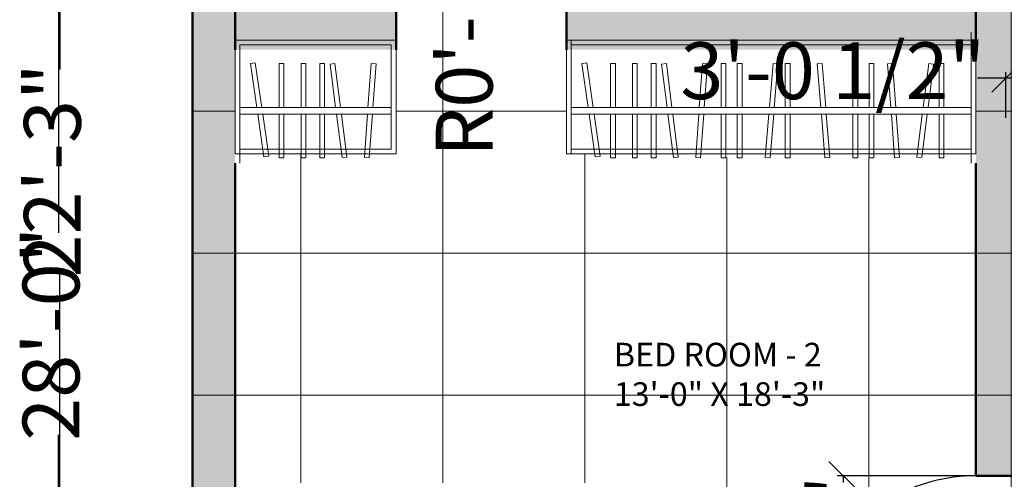
# Model space of a CAD drawing. Units: inches. Extents: x 2371 to 3019, y 129 to 700.
# Tile 3 of 14: x 2371 to 2579, y 432 to 529. Entities that reach past the tile are written whole.
import ezdxf

# ---------------------------------------------------------------- set-up
doc = ezdxf.new("R2010")
doc.units = ezdxf.units.IN
for name, color, linetype, lineweight in [('A-ANNO-DIMS', 2, 'Continuous', 18), ('A-AREA-IDEN', 7, 'Continuous', 25), ('A-DOOR', 4, 'Continuous', 25), ('A-FLOR-PATT', 252, 'Continuous', 13), ('A-FURN', 8, 'Continuous', 18), ('A-WALL', 7, 'Continuous', 50), ('A-WALL-PATT', 8, 'Continuous', 13)]:
    doc.layers.add(name, color=color, linetype=linetype, lineweight=lineweight)
doc.styles.get("Standard").update_dxf_attribs({"font": 'arial.ttf'})
doc.dimstyles.new('ISO-25', dxfattribs={"dimtxt": 12, "dimasz": 6, "dimexe": 1.25, "dimexo": 0.625, "dimtad": 0, "dimdec": 1, "dimlunit": 3, "dimtxsty": 'Standard', "dimblk": 'OBLIQUE', "dimblk1": 'ORIGIN2', "dimblk2": 'OBLIQUE', "dimcen": 2.5, "dimadec": 0, "dimazin": 0, "dimtfac": 1, "dimtdec": 1, "dimtmove": 0, "dimatfit": 3, "dimldrblk": 'OBLIQUE', "dimfxl": 1, "dimarcsym": 0})

# ---------------------------------------------------------------- blocks, each defined once
blk = doc.blocks.new('*U4')
for p, q in [((0, 0), (0, -6)), ((36, 0), (36, -6))]:
    blk.add_line(p, q)
blk.add_lwpolyline([(0, 0), (31.18, 18), (32.05, 16.48), (0.88, -1.52)], close=True)
blk.add_arc((0, 0), 36, 0, 30)
blk = doc.blocks.new('_Oblique')
at = {"color": 0, "linetype": 'ByBlock', "lineweight": -2}
blk.add_line((-0.5, -0.5), (0.5, 0.5), dxfattribs=at)
blk = doc.blocks.new('*D18')
at = {"layer": 'A-ANNO-DIMS', "color": 0, "lineweight": -2, "transparency": 16777216}
for p, q in [((2406.48, 630.98), (2377.53, 630.98)), ((2378.78, 630.98), (2378.78, 484.31)), ((2378.78, 294.98), (2378.78, 441.64)), ((2406.48, 294.98), (2377.53, 294.98))]:
    blk.add_line(p, q, dxfattribs=at)
at = {"layer": 'Defpoints', "color": 0, "lineweight": 25, "transparency": 16777216}
for p in [(2407.11, 630.98), (2378.78, 294.98), (2407.11, 294.98)]:
    blk.add_point(p, dxfattribs=at)
at = {"layer": 'A-ANNO-DIMS', "color": 0, "lineweight": -2, "transparency": 16777216, "xscale": 6, "yscale": 6, "zscale": 6}
for p, rotation in [((2378.78, 630.98), 90), ((2378.78, 294.98), 270)]:
    blk.add_blockref('_Oblique', p, dxfattribs=dict(at, rotation=rotation))
at = {"layer": 'A-ANNO-DIMS', "color": 0, "transparency": 16777216, "insert": (2378.78, 462.98), "char_height": 12, "attachment_point": 5, "rotation": 90}
blk.add_mtext('28\'-0"', dxfattribs=at)
blk = doc.blocks.new('_Origin2')
at = {"color": 0, "linetype": 'ByBlock', "lineweight": -2}
blk.add_line((-0.5, 0), (-1, 0), dxfattribs=at)
for radius in [0.5, 0.25]:
    blk.add_circle((0, 0), radius, dxfattribs=at)
blk = doc.blocks.new('*D33')
at = {"layer": 'A-ANNO-DIMS', "color": 0, "lineweight": -2, "transparency": 16777216}
for p, q in [((2578.94, 508.6), (2578.94, 518.23)), ((2615.61, 508.6), (2615.61, 518.23)), ((2578.94, 516.98), (2572.94, 516.98)), ((2615.61, 516.98), (2578.94, 516.98))]:
    blk.add_line(p, q, dxfattribs=at)
at = {"layer": 'Defpoints', "color": 0, "lineweight": 25, "transparency": 16777216}
for p in [(2578.94, 516.98), (2578.94, 507.98), (2615.61, 507.98)]:
    blk.add_point(p, dxfattribs=at)
at = {"layer": 'A-ANNO-DIMS', "color": 0, "lineweight": -2, "transparency": 16777216, "xscale": 6, "yscale": 6, "zscale": 6, "rotation": 180}
blk.add_blockref('_Oblique', (2578.94, 516.98), dxfattribs=at)
at = {"layer": 'A-ANNO-DIMS', "color": 0, "lineweight": -2, "transparency": 16777216, "xscale": 6, "yscale": 6, "zscale": 6}
blk.add_blockref('_Oblique', (2615.61, 516.98), dxfattribs=at)
at = {"layer": 'A-ANNO-DIMS', "color": 0, "transparency": 16777216, "insert": (2542.39, 516.98), "char_height": 12, "attachment_point": 5}
blk.add_mtext('3\'-0 1/2"', dxfattribs=at)
blk = doc.blocks.new('*D60')
at = {"layer": 'A-ANNO-DIMS', "color": 0, "lineweight": -2, "transparency": 16777216}
for p, q in [((2406.48, 630.98), (2377.81, 630.98)), ((2379.06, 630.98), (2379.06, 518.81)), ((2379.06, 363.98), (2379.06, 476.14)), ((2406.48, 363.98), (2377.81, 363.98))]:
    blk.add_line(p, q, dxfattribs=at)
at = {"layer": 'Defpoints', "color": 0, "lineweight": 25, "transparency": 16777216}
for p in [(2379.06, 630.98), (2407.11, 630.98), (2407.11, 363.98)]:
    blk.add_point(p, dxfattribs=at)
at = {"layer": 'A-ANNO-DIMS', "color": 0, "lineweight": -2, "transparency": 16777216, "xscale": 6, "yscale": 6, "zscale": 6}
for p, rotation in [((2379.06, 630.98), 90), ((2379.06, 363.98), 270)]:
    blk.add_blockref('_Oblique', p, dxfattribs=dict(at, rotation=rotation))
at = {"layer": 'A-ANNO-DIMS', "color": 0, "transparency": 16777216, "insert": (2379.06, 497.48), "char_height": 12, "attachment_point": 5, "rotation": 90}
blk.add_mtext('22\'-3"', dxfattribs=at)
blk = doc.blocks.new('*D70')
at = {"layer": 'A-ANNO-DIMS', "color": 0, "lineweight": -2, "transparency": 16777216}
for p, q in [((2571.98, 432.98), (2543.31, 432.98)), ((2544.56, 432.98), (2544.56, 431.55)), ((2544.56, 396.98), (2544.56, 398.41)), ((2571.98, 396.98), (2543.31, 396.98))]:
    blk.add_line(p, q, dxfattribs=at)
at = {"layer": 'Defpoints', "color": 0, "lineweight": 25, "transparency": 16777216}
for p in [(2544.56, 432.98), (2572.61, 432.98), (2572.61, 396.98)]:
    blk.add_point(p, dxfattribs=at)
at = {"layer": 'A-ANNO-DIMS', "color": 0, "lineweight": -2, "transparency": 16777216, "xscale": 6, "yscale": 6, "zscale": 6}
for p, rotation in [((2544.56, 432.98), 90), ((2544.56, 396.98), 270)]:
    blk.add_blockref('_Oblique', p, dxfattribs=dict(at, rotation=rotation))
at = {"layer": 'A-ANNO-DIMS', "color": 0, "transparency": 16777216, "insert": (2544.56, 414.98), "char_height": 12, "attachment_point": 5, "rotation": 90}
blk.add_mtext('3\'-0"', dxfattribs=at)
blk = doc.blocks.new('*D76')
at = {"layer": 'A-ANNO-DIMS', "color": 0, "lineweight": -2, "transparency": 16777216}
for p, q in [((2450.11, 523.6), (2450.11, 552.28)), ((2486.11, 523.6), (2486.11, 552.28)), ((2450.11, 551.03), (2451.53, 551.03)), ((2486.11, 551.03), (2484.68, 551.03))]:
    blk.add_line(p, q, dxfattribs=at)
at = {"layer": 'Defpoints', "color": 0, "lineweight": 25, "transparency": 16777216}
for p in [(2486.11, 551.03), (2450.11, 522.98), (2486.11, 522.98)]:
    blk.add_point(p, dxfattribs=at)
at = {"layer": 'A-ANNO-DIMS', "color": 0, "lineweight": -2, "transparency": 16777216, "xscale": 6, "yscale": 6, "zscale": 6, "rotation": 180}
blk.add_blockref('_Oblique', (2450.11, 551.03), dxfattribs=at)
at = {"layer": 'A-ANNO-DIMS', "color": 0, "lineweight": -2, "transparency": 16777216, "xscale": 6, "yscale": 6, "zscale": 6}
blk.add_blockref('_Oblique', (2486.11, 551.03), dxfattribs=at)
at = {"layer": 'A-ANNO-DIMS', "color": 0, "transparency": 16777216, "insert": (2468.11, 551.03), "char_height": 12, "attachment_point": 5}
blk.add_mtext('3\'-0"', dxfattribs=at)
blk = doc.blocks.new('*D81')
at = {"layer": 'A-ANNO-DIMS', "color": 0, "lineweight": -2, "transparency": 16777216}
for p in [(2466.11, 605.98), (2466.09, 583.23)]:
    blk.add_line(p, (2466.1, 595.23), dxfattribs=at)
at = {"layer": 'Defpoints', "color": 0, "lineweight": 25, "transparency": 16777216}
for p in [(2466.11, 605.98), (2466.1, 595.23)]:
    blk.add_point(p, dxfattribs=at)
at = {"layer": 'A-ANNO-DIMS', "color": 0, "lineweight": -2, "transparency": 16777216, "xscale": 6, "yscale": 6, "zscale": 6, "rotation": 89.97280933984025}
blk.add_blockref('_Oblique', (2466.1, 595.23), dxfattribs=at)
at = {"layer": 'A-ANNO-DIMS', "color": 0, "transparency": 16777216, "insert": (2466.07, 542.27), "char_height": 12, "attachment_point": 5, "rotation": 89.9728}
blk.add_mtext('R0\'-10 1/2"', dxfattribs=at)

msp = doc.modelspace()

# ---------------------------------------------------------------- hatches: boundary and pattern name
at = {"layer": 'A-FLOR-PATT'}
h = msp.add_hatch(dxfattribs=at)
h.set_pattern_fill('_USER', color=256, scale=30, pattern_type=0)
h.set_pattern_definition([(0, (0, 0), (0, 30), [])])
h.paths.add_polyline_path([(2913.11, 498.98), (2827.61, 498.98), (2827.61, 531.98), (2832.11, 531.98), (2832.11, 537.98), (2833.61, 537.98), (2833.61, 605.98), (2818.35, 605.98, -1), (2796.86, 605.98), (2781.61, 605.98), (2781.61, 603.98), (2781.61, 533.98), (2757.61, 533.98), (2757.61, 531.98), (2797.61, 531.98), (2797.61, 522.98), (2757.61, 522.98), (2757.61, 516.98), (2754.59, 516.98), (2772.52, 485.76), (2771.01, 484.89), (2770.98, 484.93, -0.097552), (2757.61, 481.1), (2757.61, 422.48), (2837.61, 422.48), (2837.61, 362.48), (2757.61, 362.48), (2757.61, 303.98), (2835.86, 303.98, -0.09439), (2793.86, 311.98), (2793.86, 337.98), (2799.86, 337.98), (2799.86, 336.42), (2871.86, 336.42), (2871.86, 337.98), (2877.86, 337.98), (2877.86, 311.98, -0.09439), (2835.86, 303.98), (2913.11, 303.98), (2913.11, 383.18), (2904.11, 383.18), (2904.11, 419.18), (2913.11, 419.18)])
h.paths.add_polyline_path([(2788.88, 332.88), (2788.88, 308.88), (2764.88, 308.88), (2764.88, 332.88)], flags=16)
h.paths.add_polyline_path([(2788.4, 325.04, -1), (2774.4, 325.04, -1)], flags=0)
h.paths.add_polyline_path([(2781.4, 328.04), (2784.4, 325.04), (2781.4, 322.04), (2778.4, 325.04)], flags=0)
h.paths.add_polyline_path([(2782.4, 325.04, -1), (2780.4, 325.04, -1)], flags=0)
h.paths.add_polyline_path([(2748.61, 480.99), (2754.51, 480.98, 0.119303), (2770.98, 484.93), (2753.07, 516.1), (2754.59, 516.98), (2748.61, 516.98), (2748.61, 539.98), (2712.61, 539.98), (2665.11, 539.98, -0.09439), (2707.11, 531.98), (2707.11, 505.98), (2701.11, 505.98), (2701.11, 507.53), (2629.11, 507.53), (2629.11, 505.98), (2623.11, 505.98), (2623.11, 531.98, -0.09439), (2665.11, 539.98), (2581.61, 539.98), (2581.61, 522.98), (2581.61, 477.98, -0.131044), (2589.61, 507.98), (2615.61, 507.98), (2615.61, 501.98), (2614.05, 501.98), (2614.05, 453.98), (2615.61, 453.98), (2615.61, 447.98), (2589.61, 447.98, -0.131044), (2581.61, 477.98), (2581.61, 432.98), (2572.61, 432.98, 0.119303), (2556.14, 428.99), (2574.12, 397.85), (2572.61, 396.98), (2578.61, 396.98), (2581.61, 396.98), (2581.61, 390.98), (2748.61, 390.98)])
h.paths.add_polyline_path([(2683.1, 447.25), (2652.43, 447.25), (2652.43, 492.22), (2683.1, 492.22)], flags=16)
h.paths.add_polyline_path([(2682.1, 448.25), (2653.43, 448.25), (2653.43, 491.22), (2682.1, 491.22)], flags=0)
h.paths.add_polyline_path([(2613.58, 512.06), (2589.58, 512.06), (2589.58, 536.06), (2613.58, 536.06)], flags=16)
h.paths.add_polyline_path([(2599.1, 528.22, -1), (2613.1, 528.22, -1)], flags=0)
h.paths.add_polyline_path([(2609.1, 528.22), (2606.1, 525.22), (2603.1, 528.22), (2606.1, 531.22)], flags=0)
h.paths.add_polyline_path([(2607.1, 528.22, -1), (2605.1, 528.22, -1)], flags=0)
h.paths.add_polyline_path([(2581.61, 522.98), (2581.61, 621.98), (2572.61, 621.98), (2572.61, 522.98), (2572.61, 500.98), (2565.85, 500.98), (2565.85, 500.15), (2564.82, 500.15), (2561.16, 500.19), (2561.16, 500.17), (2560.13, 500.3), (2560.22, 500.98), (2556.38, 500.98), (2556.43, 500.22), (2555.4, 500.14), (2555.34, 500.98), (2551.07, 500.98), (2551.07, 500.15), (2550.04, 500.15), (2547.64, 500.19), (2547.64, 500.15), (2546.61, 500.15), (2541.79, 500.22), (2540.72, 500.13), (2540.65, 500.98), (2533.37, 500.98), (2533.37, 500.15), (2532.34, 500.15), (2529.13, 500.21), (2529.12, 500.13), (2528.09, 500.22), (2528.16, 500.98), (2523.23, 500.98), (2523.23, 500.15), (2522.2, 500.15), (2519.8, 500.21), (2519.8, 500.15), (2518.77, 500.15), (2514.45, 500.26), (2514.44, 500.14), (2513.41, 500.22), (2513.47, 500.98), (2509.62, 500.98), (2509.71, 500.3), (2508.69, 500.17), (2508.58, 500.98), (2505.03, 500.98), (2505.03, 500.15), (2503.99, 500.15), (2501.07, 500.29), (2501.07, 500.15), (2500.04, 500.15), (2496.44, 500.37), (2496.44, 500.15), (2495.4, 500.15), (2492.55, 500.41), (2492.18, 500.35), (2492.09, 500.98), (2486.11, 500.98), (2486.11, 524.98), (2486.11, 531.98), (2490.61, 531.98), (2490.61, 537.98), (2492.11, 537.98), (2492.11, 605.98), (2476.85, 605.98, -1), (2455.36, 605.98), (2440.11, 605.98), (2440.11, 533.98), (2416.11, 533.98), (2416.11, 605.98), (2416.11, 621.98), (2536.61, 621.98), (2536.61, 630.98), (2407.11, 630.98), (2407.11, 363.98), (2416.11, 363.98), (2416.11, 431.48), (2496.11, 431.48), (2496.11, 371.48), (2416.11, 371.48), (2416.11, 303.98), (2494.36, 303.98, -0.09439), (2452.36, 311.98), (2452.36, 337.98), (2458.36, 337.98), (2458.36, 336.42), (2530.36, 336.42), (2530.36, 337.98), (2536.36, 337.98), (2536.36, 311.98, -0.09439), (2494.36, 303.98), (2572.61, 303.98), (2572.61, 381.98), (2572.61, 396.98), (2554.61, 428.15), (2556.12, 429.03), (2556.14, 428.99, -0.119303), (2572.61, 432.98), (2578.61, 432.98), (2581.61, 432.98)])
h.paths.add_polyline_path([(2450.11, 500.98), (2444.5, 500.98), (2444.44, 500.14), (2443.41, 500.22), (2443.47, 500.98), (2439.62, 500.98), (2439.71, 500.3), (2438.69, 500.17), (2438.58, 500.98), (2435.02, 500.98), (2435.02, 500.15), (2433.99, 500.15), (2433.99, 500.98), (2431.07, 500.98), (2431.07, 500.15), (2430.04, 500.15), (2430.04, 500.98), (2426.43, 500.98), (2426.43, 500.15), (2425.4, 500.15), (2425.4, 500.98), (2423.13, 500.98), (2423.2, 500.5), (2422.18, 500.35), (2422.09, 500.98), (2416.11, 500.98), (2416.11, 524.98), (2416.11, 531.98), (2450.11, 531.98), (2450.11, 522.98)], flags=16)
h.paths.add_polyline_path([(2449.11, 501.98), (2417.11, 501.98), (2417.11, 522.98), (2417.11, 523.98), (2449.11, 523.98)], flags=0)
h.paths.add_polyline_path([(2420.7, 510.73), (2419.36, 520.07), (2420.38, 520.22), (2421.74, 510.73), (2425.4, 510.73), (2425.4, 520.07), (2426.43, 520.07), (2426.43, 510.73), (2430.04, 510.73), (2430.04, 520.07), (2431.07, 520.07), (2431.07, 510.73), (2433.99, 510.73), (2433.99, 520.07), (2435.02, 520.07), (2435.02, 510.73), (2437.35, 510.73), (2436.18, 519.93), (2437.2, 520.06), (2438.39, 510.73), (2444.17, 510.73), (2444.85, 520.08), (2445.88, 520.01), (2445.21, 510.73)], flags=0)
h.paths.add_polyline_path([(2446.94, 336.11), (2446.94, 312.11), (2422.94, 312.11), (2422.94, 336.11)], flags=16)
h.paths.add_polyline_path([(2446.46, 328.27, -1), (2432.46, 328.27, -1)], flags=0)
h.paths.add_polyline_path([(2439.46, 331.27), (2442.46, 328.27), (2439.46, 325.27), (2436.46, 328.27)], flags=0)
h.paths.add_polyline_path([(2440.46, 328.27, -1), (2438.46, 328.27, -1)], flags=0)
h.paths.add_polyline_path([(2816, 444.88), (2866.87, 444.88), (2866.87, 463.54), (2816, 463.54)], flags=24)
h.paths.add_polyline_path([(2794.21, 558.3), (2833.34, 558.3), (2833.34, 576.96), (2794.21, 576.96)], flags=24)
h.paths.add_polyline_path([(2651.69, 411.53), (2711.04, 411.53), (2711.04, 430.19), (2651.69, 430.19)], flags=24)
h.paths.add_polyline_path([(2494.09, 444.88), (2544.97, 444.88), (2544.97, 463.54), (2494.09, 463.54)], flags=24)
h.paths.add_polyline_path([(2444.55, 565.02), (2483.69, 565.02), (2483.69, 583.68), (2444.55, 583.68)], flags=24)
h = msp.add_hatch(dxfattribs=at)
h.set_pattern_fill('_USER', color=256, scale=30, angle=90, pattern_type=0)
h.set_pattern_definition([(90, (0, 0), (-30, 2e-15), [])])
h.paths.add_polyline_path([(2913.11, 498.98), (2827.61, 498.98), (2827.61, 531.98), (2832.11, 531.98), (2832.11, 537.98), (2833.61, 537.98), (2833.61, 605.98), (2818.35, 605.98, -1), (2796.86, 605.98), (2781.61, 605.98), (2781.61, 603.98), (2781.61, 533.98), (2757.61, 533.98), (2757.61, 531.98), (2797.61, 531.98), (2797.61, 522.98), (2757.61, 522.98), (2757.61, 516.98), (2754.59, 516.98), (2772.52, 485.76), (2771.01, 484.89), (2770.98, 484.93, -0.097552), (2757.61, 481.1), (2757.61, 422.48), (2837.61, 422.48), (2837.61, 362.48), (2757.61, 362.48), (2757.61, 303.98), (2835.86, 303.98, -0.09439), (2793.86, 311.98), (2793.86, 337.98), (2799.86, 337.98), (2799.86, 336.42), (2871.86, 336.42), (2871.86, 337.98), (2877.86, 337.98), (2877.86, 311.98, -0.09439), (2835.86, 303.98), (2913.11, 303.98), (2913.11, 383.18), (2904.11, 383.18), (2904.11, 419.18), (2913.11, 419.18)])
h.paths.add_polyline_path([(2788.88, 332.88), (2788.88, 308.88), (2764.88, 308.88), (2764.88, 332.88)], flags=16)
h.paths.add_polyline_path([(2788.4, 325.04, -1), (2774.4, 325.04, -1)], flags=0)
h.paths.add_polyline_path([(2781.4, 328.04), (2784.4, 325.04), (2781.4, 322.04), (2778.4, 325.04)], flags=0)
h.paths.add_polyline_path([(2782.4, 325.04, -1), (2780.4, 325.04, -1)], flags=0)
h.paths.add_polyline_path([(2748.61, 480.99), (2754.51, 480.98, 0.119303), (2770.98, 484.93), (2753.07, 516.1), (2754.59, 516.98), (2748.61, 516.98), (2748.61, 539.98), (2712.61, 539.98), (2665.11, 539.98, -0.09439), (2707.11, 531.98), (2707.11, 505.98), (2701.11, 505.98), (2701.11, 507.53), (2629.11, 507.53), (2629.11, 505.98), (2623.11, 505.98), (2623.11, 531.98, -0.09439), (2665.11, 539.98), (2581.61, 539.98), (2581.61, 522.98), (2581.61, 477.98, -0.131044), (2589.61, 507.98), (2615.61, 507.98), (2615.61, 501.98), (2614.05, 501.98), (2614.05, 453.98), (2615.61, 453.98), (2615.61, 447.98), (2589.61, 447.98, -0.131044), (2581.61, 477.98), (2581.61, 432.98), (2572.61, 432.98, 0.119303), (2556.14, 428.99), (2574.12, 397.85), (2572.61, 396.98), (2578.61, 396.98), (2581.61, 396.98), (2581.61, 390.98), (2748.61, 390.98)])
h.paths.add_polyline_path([(2683.1, 447.25), (2652.43, 447.25), (2652.43, 492.22), (2683.1, 492.22)], flags=16)
h.paths.add_polyline_path([(2682.1, 448.25), (2653.43, 448.25), (2653.43, 491.22), (2682.1, 491.22)], flags=0)
h.paths.add_polyline_path([(2613.58, 512.06), (2589.58, 512.06), (2589.58, 536.06), (2613.58, 536.06)], flags=16)
h.paths.add_polyline_path([(2599.1, 528.22, -1), (2613.1, 528.22, -1)], flags=0)
h.paths.add_polyline_path([(2609.1, 528.22), (2606.1, 525.22), (2603.1, 528.22), (2606.1, 531.22)], flags=0)
h.paths.add_polyline_path([(2607.1, 528.22, -1), (2605.1, 528.22, -1)], flags=0)
h.paths.add_polyline_path([(2581.61, 522.98), (2581.61, 621.98), (2572.61, 621.98), (2572.61, 522.98), (2572.61, 500.98), (2565.85, 500.98), (2565.85, 500.15), (2564.82, 500.15), (2561.16, 500.19), (2561.16, 500.17), (2560.13, 500.3), (2560.22, 500.98), (2556.38, 500.98), (2556.43, 500.22), (2555.4, 500.14), (2555.34, 500.98), (2551.07, 500.98), (2551.07, 500.15), (2550.04, 500.15), (2547.64, 500.19), (2547.64, 500.15), (2546.61, 500.15), (2541.79, 500.22), (2540.72, 500.13), (2540.65, 500.98), (2533.37, 500.98), (2533.37, 500.15), (2532.34, 500.15), (2529.13, 500.21), (2529.12, 500.13), (2528.09, 500.22), (2528.16, 500.98), (2523.23, 500.98), (2523.23, 500.15), (2522.2, 500.15), (2519.8, 500.21), (2519.8, 500.15), (2518.77, 500.15), (2514.45, 500.26), (2514.44, 500.14), (2513.41, 500.22), (2513.47, 500.98), (2509.62, 500.98), (2509.71, 500.3), (2508.69, 500.17), (2508.58, 500.98), (2505.03, 500.98), (2505.03, 500.15), (2503.99, 500.15), (2501.07, 500.29), (2501.07, 500.15), (2500.04, 500.15), (2496.44, 500.37), (2496.44, 500.15), (2495.4, 500.15), (2492.55, 500.41), (2492.18, 500.35), (2492.09, 500.98), (2486.11, 500.98), (2486.11, 524.98), (2486.11, 531.98), (2490.61, 531.98), (2490.61, 537.98), (2492.11, 537.98), (2492.11, 605.98), (2476.85, 605.98, -1), (2455.36, 605.98), (2440.11, 605.98), (2440.11, 533.98), (2416.11, 533.98), (2416.11, 605.98), (2416.11, 621.98), (2536.61, 621.98), (2536.61, 630.98), (2407.11, 630.98), (2407.11, 363.98), (2416.11, 363.98), (2416.11, 431.48), (2496.11, 431.48), (2496.11, 371.48), (2416.11, 371.48), (2416.11, 303.98), (2494.36, 303.98, -0.09439), (2452.36, 311.98), (2452.36, 337.98), (2458.36, 337.98), (2458.36, 336.42), (2530.36, 336.42), (2530.36, 337.98), (2536.36, 337.98), (2536.36, 311.98, -0.09439), (2494.36, 303.98), (2572.61, 303.98), (2572.61, 381.98), (2572.61, 396.98), (2554.61, 428.15), (2556.12, 429.03), (2556.14, 428.99, -0.119303), (2572.61, 432.98), (2578.61, 432.98), (2581.61, 432.98)])
h.paths.add_polyline_path([(2450.11, 500.98), (2444.5, 500.98), (2444.44, 500.14), (2443.41, 500.22), (2443.47, 500.98), (2439.62, 500.98), (2439.71, 500.3), (2438.69, 500.17), (2438.58, 500.98), (2435.02, 500.98), (2435.02, 500.15), (2433.99, 500.15), (2433.99, 500.98), (2431.07, 500.98), (2431.07, 500.15), (2430.04, 500.15), (2430.04, 500.98), (2426.43, 500.98), (2426.43, 500.15), (2425.4, 500.15), (2425.4, 500.98), (2423.13, 500.98), (2423.2, 500.5), (2422.18, 500.35), (2422.09, 500.98), (2416.11, 500.98), (2416.11, 524.98), (2416.11, 531.98), (2450.11, 531.98), (2450.11, 522.98)], flags=16)
h.paths.add_polyline_path([(2449.11, 501.98), (2417.11, 501.98), (2417.11, 522.98), (2417.11, 523.98), (2449.11, 523.98)], flags=0)
h.paths.add_polyline_path([(2420.7, 510.73), (2419.36, 520.07), (2420.38, 520.22), (2421.74, 510.73), (2425.4, 510.73), (2425.4, 520.07), (2426.43, 520.07), (2426.43, 510.73), (2430.04, 510.73), (2430.04, 520.07), (2431.07, 520.07), (2431.07, 510.73), (2433.99, 510.73), (2433.99, 520.07), (2435.02, 520.07), (2435.02, 510.73), (2437.35, 510.73), (2436.18, 519.93), (2437.2, 520.06), (2438.39, 510.73), (2444.17, 510.73), (2444.85, 520.08), (2445.88, 520.01), (2445.21, 510.73)], flags=0)
h.paths.add_polyline_path([(2446.94, 336.11), (2446.94, 312.11), (2422.94, 312.11), (2422.94, 336.11)], flags=16)
h.paths.add_polyline_path([(2446.46, 328.27, -1), (2432.46, 328.27, -1)], flags=0)
h.paths.add_polyline_path([(2439.46, 331.27), (2442.46, 328.27), (2439.46, 325.27), (2436.46, 328.27)], flags=0)
h.paths.add_polyline_path([(2440.46, 328.27, -1), (2438.46, 328.27, -1)], flags=0)
h.paths.add_polyline_path([(2816, 444.88), (2866.87, 444.88), (2866.87, 463.54), (2816, 463.54)], flags=24)
h.paths.add_polyline_path([(2794.21, 558.3), (2833.34, 558.3), (2833.34, 576.96), (2794.21, 576.96)], flags=24)
h.paths.add_polyline_path([(2651.69, 411.53), (2711.04, 411.53), (2711.04, 430.19), (2651.69, 430.19)], flags=24)
h.paths.add_polyline_path([(2494.09, 444.88), (2544.97, 444.88), (2544.97, 463.54), (2494.09, 463.54)], flags=24)
h.paths.add_polyline_path([(2444.55, 565.02), (2483.69, 565.02), (2483.69, 583.68), (2444.55, 583.68)], flags=24)
at = {"layer": 'A-WALL-PATT'}
h = msp.add_hatch(color=256, dxfattribs=at)
h.dxf.hatch_style = 1
h.paths.add_polyline_path([(2536.61, 630.98), (2407.11, 630.98), (2407.11, 363.98), (2416.11, 363.98), (2416.11, 498.98), (2416.11, 522.98), (2416.11, 531.98), (2416.11, 603.98), (2416.11, 621.98), (2536.61, 621.98)])
h.paths.add_polyline_path([(2630.98, 630.98), (2560.61, 630.98), (2560.61, 621.98), (2630.98, 621.98)])
h.paths.add_polyline_path([(2878.11, 630.98), (2699.23, 630.98), (2699.23, 621.98), (2878.11, 621.98)])
h.paths.add_polyline_path([(2496.61, 621.98), (2492.11, 621.98), (2492.11, 569.98), (2496.61, 569.98)], flags=17)
h.paths.add_polyline_path([(2581.61, 621.98), (2572.61, 621.98), (2572.61, 522.98), (2572.61, 498.98), (2572.61, 432.98), (2578.61, 432.98), (2581.61, 432.98), (2581.61, 522.98)])
h.paths.add_polyline_path([(2572.61, 531.98), (2486.11, 531.98), (2486.11, 522.98), (2572.61, 522.98)])
h.paths.add_polyline_path([(2450.11, 531.98), (2440.11, 531.98), (2416.11, 531.98), (2416.11, 522.98), (2450.11, 522.98)], flags=17)
h.paths.add_polyline_path([(2416.11, 315.98), (2407.11, 315.98), (2407.11, 294.98), (2458.11, 294.98), (2458.11, 303.98), (2416.11, 303.98)])
h.paths.add_polyline_path([(2757.61, 303.98), (2530.61, 303.98), (2530.61, 294.98), (2757.61, 294.98)])
h.paths.add_polyline_path([(2581.61, 381.98), (2605.61, 381.98), (2617.61, 381.98), (2617.61, 390.98), (2581.61, 390.98), (2581.61, 396.98), (2572.61, 396.98), (2572.61, 381.98), (2572.61, 303.98), (2581.61, 303.98)])
h.paths.add_polyline_path([(2757.61, 480.98), (2748.61, 480.98), (2748.61, 381.98), (2748.61, 303.98), (2757.61, 303.98), (2757.61, 381.98), (2757.61, 422.48)])
h.paths.add_polyline_path([(2797.61, 531.98), (2757.61, 531.98), (2757.61, 603.98), (2757.61, 621.98), (2748.61, 621.98), (2748.61, 516.99), (2754.59, 516.98), (2757.61, 516.98), (2757.61, 522.98), (2797.61, 522.98)])
h.paths.add_polyline_path([(2913.11, 531.98), (2827.61, 531.98), (2827.61, 522.98), (2913.11, 522.98)])
h.paths.add_polyline_path([(2923.11, 630.98), (2902.11, 630.98), (2902.11, 621.98), (2914.11, 621.98), (2914.11, 363.98), (2923.11, 363.98)])
h.paths.add_polyline_path([(2923.11, 315.98), (2914.11, 315.98), (2914.11, 303.98), (2866.11, 303.98), (2866.11, 294.98), (2923.11, 294.98)])
h.paths.add_polyline_path([(2793.61, 303.98), (2757.61, 303.98), (2757.61, 294.98), (2793.61, 294.98)])

# ---------------------------------------------------------------- linework, layer by layer
at = {"layer": 'A-FURN'}
for p, q in [((2487.11, 500.98), (2487.11, 524.98)), ((2571.61, 525.62), (2571.61, 498.98)), ((2417.11, 498.98), (2417.11, 522.98)), ((2449.11, 510.73), (2417.16, 510.73)), ((2501.61, 510.73), (2487.11, 510.73)), ((2571.61, 510.73), (2487.16, 510.73)), ((2417.16, 509.33), (2449.11, 509.33)), ((2487.11, 509.33), (2501.61, 509.33)), ((2487.16, 509.33), (2571.61, 509.33))]:
    msp.add_line(p, q, dxfattribs=at)
for points in [[(2571.61, 526.65), (2571.61, 525.62)], [(2421.74, 510.73), (2420.38, 520.22), (2419.36, 520.07), (2420.7, 510.73)], [(2426.43, 510.73), (2426.43, 520.07), (2425.4, 520.07), (2425.4, 510.73)], [(2431.07, 510.73), (2431.07, 520.07), (2430.04, 520.07), (2430.04, 510.73)], [(2435.02, 510.73), (2435.02, 520.07), (2433.99, 520.07), (2433.99, 510.73)], [(2438.39, 510.73), (2437.2, 520.06), (2436.18, 519.93), (2437.35, 510.73)], [(2445.21, 510.73), (2445.88, 520.01), (2444.85, 520.08), (2444.17, 510.73)], [(2491.74, 510.73), (2490.38, 520.22), (2489.36, 520.07), (2490.7, 510.73)], [(2496.44, 510.73), (2496.44, 520.07), (2495.4, 520.07), (2495.4, 510.73)], [(2501.07, 510.73), (2501.07, 520.07), (2500.04, 520.07), (2500.04, 510.73)], [(2505.03, 510.73), (2505.03, 520.07), (2503.99, 520.07), (2503.99, 510.73)], [(2508.39, 510.73), (2507.21, 520.06), (2506.18, 519.93), (2507.35, 510.73)], [(2515.21, 510.73), (2515.88, 520.01), (2514.85, 520.08), (2514.17, 510.73)], [(2519.8, 510.73), (2519.8, 520.07), (2518.77, 520.07), (2518.77, 510.73)], [(2523.23, 510.73), (2523.23, 520.07), (2522.2, 520.07), (2522.2, 510.73)], [(2530, 510.73), (2530.77, 519.98), (2529.75, 520.07), (2528.97, 510.73)], [(2533.37, 510.73), (2533.37, 520.07), (2532.34, 520.07), (2532.34, 510.73)], [(2539.84, 510.73), (2539.07, 519.98), (2540.1, 520.07), (2540.87, 510.73)], [(2546.61, 510.73), (2546.61, 520.07), (2547.64, 520.07), (2547.64, 510.73)], [(2550.04, 510.73), (2550.04, 520.07), (2551.07, 520.07), (2551.07, 510.73)], [(2554.64, 510.73), (2553.96, 520.01), (2554.99, 520.08), (2555.67, 510.73)], [(2561.46, 510.73), (2562.64, 520.06), (2563.66, 519.93), (2562.49, 510.73)], [(2564.82, 510.73), (2564.82, 520.07), (2565.85, 520.07), (2565.85, 510.73)], [(2420.9, 509.33), (2422.18, 500.35), (2423.2, 500.5)], [(2423.2, 500.5), (2421.94, 509.33)], [(2425.4, 509.33), (2425.4, 500.15), (2426.43, 500.15)], [(2426.43, 500.15), (2426.43, 509.33)], [(2430.04, 509.33), (2430.04, 500.15), (2431.07, 500.15)], [(2431.07, 500.15), (2431.07, 509.33)], [(2433.99, 509.33), (2433.99, 500.15), (2435.02, 500.15)], [(2435.02, 500.15), (2435.02, 509.33)], [(2437.52, 509.33), (2438.69, 500.17), (2439.71, 500.3)], [(2439.71, 500.3), (2438.56, 509.33)], [(2444.07, 509.33), (2443.41, 500.22), (2444.44, 500.14)], [(2444.44, 500.14), (2445.1, 509.33)], [(2490.9, 509.33), (2492.18, 500.35), (2493.2, 500.5)], [(2493.2, 500.5), (2491.94, 509.33)], [(2495.4, 509.33), (2495.4, 500.15), (2496.44, 500.15)], [(2496.44, 500.15), (2496.44, 509.33)], [(2500.04, 509.33), (2500.04, 500.15), (2501.07, 500.15)], [(2501.07, 500.15), (2501.07, 509.33)], [(2503.99, 509.33), (2503.99, 500.15), (2505.03, 500.15)], [(2505.03, 500.15), (2505.03, 509.33)], [(2507.53, 509.33), (2508.69, 500.17), (2509.71, 500.3)], [(2509.71, 500.3), (2508.56, 509.33)], [(2514.07, 509.33), (2513.41, 500.22), (2514.44, 500.14)], [(2514.44, 500.14), (2515.11, 509.33)], [(2518.77, 509.33), (2518.77, 500.15), (2519.8, 500.15)], [(2519.8, 500.15), (2519.8, 509.33)], [(2522.2, 509.33), (2522.2, 500.15), (2523.23, 500.15)], [(2523.23, 500.15), (2523.23, 509.33)], [(2528.85, 509.33), (2528.09, 500.22), (2529.12, 500.13)], [(2529.12, 500.13), (2529.89, 509.33)], [(2532.34, 509.33), (2532.34, 500.15), (2533.37, 500.15)], [(2533.37, 500.15), (2533.37, 509.33)], [(2540.72, 500.13), (2539.96, 509.33)], [(2540.99, 509.33), (2541.75, 500.22), (2540.72, 500.13)], [(2546.61, 500.15), (2546.61, 509.33)], [(2547.64, 509.33), (2547.64, 500.15), (2546.61, 500.15)], [(2551.07, 509.33), (2551.07, 500.15), (2550.04, 500.15)], [(2550.04, 500.15), (2550.04, 509.33)], [(2555.4, 500.14), (2554.74, 509.33)], [(2555.77, 509.33), (2556.43, 500.22), (2555.4, 500.14)], [(2562.32, 509.33), (2561.16, 500.17), (2560.13, 500.3)], [(2560.13, 500.3), (2561.28, 509.33)], [(2565.85, 509.33), (2565.85, 500.15), (2564.82, 500.15)], [(2564.82, 500.15), (2564.82, 509.33)]]:
    msp.add_lwpolyline(points, dxfattribs=at)
for points in [[(2450.11, 524.98), (2450.11, 500.98), (2416.11, 500.98), (2416.11, 524.98)], [(2486.11, 524.98), (2486.11, 500.98), (2572.61, 500.98), (2572.61, 524.98)], [(2449.11, 523.98), (2449.11, 501.98), (2417.11, 501.98), (2417.11, 523.98)], [(2487.11, 523.98), (2487.11, 501.98), (2571.61, 501.98), (2571.61, 523.98)]]:
    msp.add_lwpolyline(points, close=True, dxfattribs=at)
at = {"layer": 'A-WALL'}
for p, q in [((2407.11, 630.98), (2407.11, 294.98)), ((2572.61, 621.98), (2572.61, 522.98)), ((2416.11, 531.98), (2416.11, 522.98)), ((2450.11, 531.98), (2450.11, 522.98)), ((2486.11, 531.98), (2486.11, 522.98)), ((2416.11, 498.98), (2416.11, 303.98)), ((2572.61, 498.98), (2572.61, 432.98)), ((2572.61, 432.98), (2581.61, 432.98))]:
    msp.add_line(p, q, dxfattribs=at)

# ---------------------------------------------------------------- block references
at = {"layer": 'A-DOOR', "rotation": 90}
msp.add_blockref('*U4', (2572.61, 396.98), dxfattribs=at)

# ---------------------------------------------------------------- texts
at = {"layer": 'A-AREA-IDEN', "ltscale": 2, "insert": (2496.11, 461.06), "char_height": 5, "attachment_point": 1}
msp.add_mtext_dynamic_manual_height_columns('BED ROOM - 2\\P13\'-0" X 18\'-3"', width=49.6634, gutter_width=12.5, heights=[0], dxfattribs=at)

# ---------------------------------------------------------------- dimensions: what is measured, and where the dimension line sits
at = {"layer": 'A-ANNO-DIMS'}
dim = msp.add_linear_dim(base=(2378.78, 294.98), p1=(2407.11, 630.98), p2=(2407.11, 294.98), angle=90, text='28\'-0"', dimstyle='ISO-25', override={"dimclrd": 0, "dimclre": 0, "dimclrt": 0}, dxfattribs=at)
dim.commit()
dim.dimension.update_dxf_attribs({"geometry": '*D18', "text_midpoint": (2378.78, 462.98)})
for base, p1, p2, angle, override, picture, middle in [((2379.06, 630.98), (2407.11, 363.98), (2407.11, 630.98), 90, {"dimdec": 1, "dimlfac": 1, "dimrnd": 0, "dimzin": 1, "dimdsep": 46, "dimlunit": 4, "dimfrac": 2}, '*D60', (2379.06, 497.48)), ((2578.94, 516.98), (2615.61, 507.98), (2578.94, 507.98), 180, {"dimdec": 1, "dimrnd": 0, "dimzin": 1, "dimlunit": 4, "dimfrac": 2}, '*D33', (2542.39, 516.98)), ((2544.56, 432.98), (2572.61, 396.98), (2572.61, 432.98), 90, {"dimdec": 1, "dimlfac": 1, "dimrnd": 0, "dimzin": 1, "dimdsep": 46, "dimlunit": 4, "dimfrac": 2}, '*D70', (2544.56, 414.98))]:
    dim = msp.add_linear_dim(base=base, p1=p1, p2=p2, angle=angle, dimstyle='ISO-25', override=override, dxfattribs=at)
    dim.commit()
    dim.dimension.update_dxf_attribs({"geometry": picture, "text_midpoint": middle})
dim = msp.add_radius_dim(center=(2466.1051, 605.9762), mpoint=(2466.1, 595.2295), dimstyle='ISO-25', override={"dimdec": 1, "dimlfac": 1, "dimrnd": 0, "dimzin": 1, "dimdsep": 46, "dimlunit": 4, "dimfrac": 2}, dxfattribs=at)
dim.commit()
dim.dimension.update_dxf_attribs({"geometry": '*D81', "text_midpoint": (2466.0749, 542.2703)})
dim = msp.add_linear_dim(base=(2486.11, 551.03), p1=(2450.11, 522.98), p2=(2486.11, 522.98), dimstyle='ISO-25', override={"dimdec": 1, "dimlfac": 1, "dimrnd": 0, "dimzin": 1, "dimdsep": 46, "dimlunit": 4, "dimfrac": 2}, dxfattribs=at)
dim.commit()
dim.dimension.update_dxf_attribs({"geometry": '*D76', "text_midpoint": (2468.11, 551.03)})

doc.saveas('drawing.dxf')
